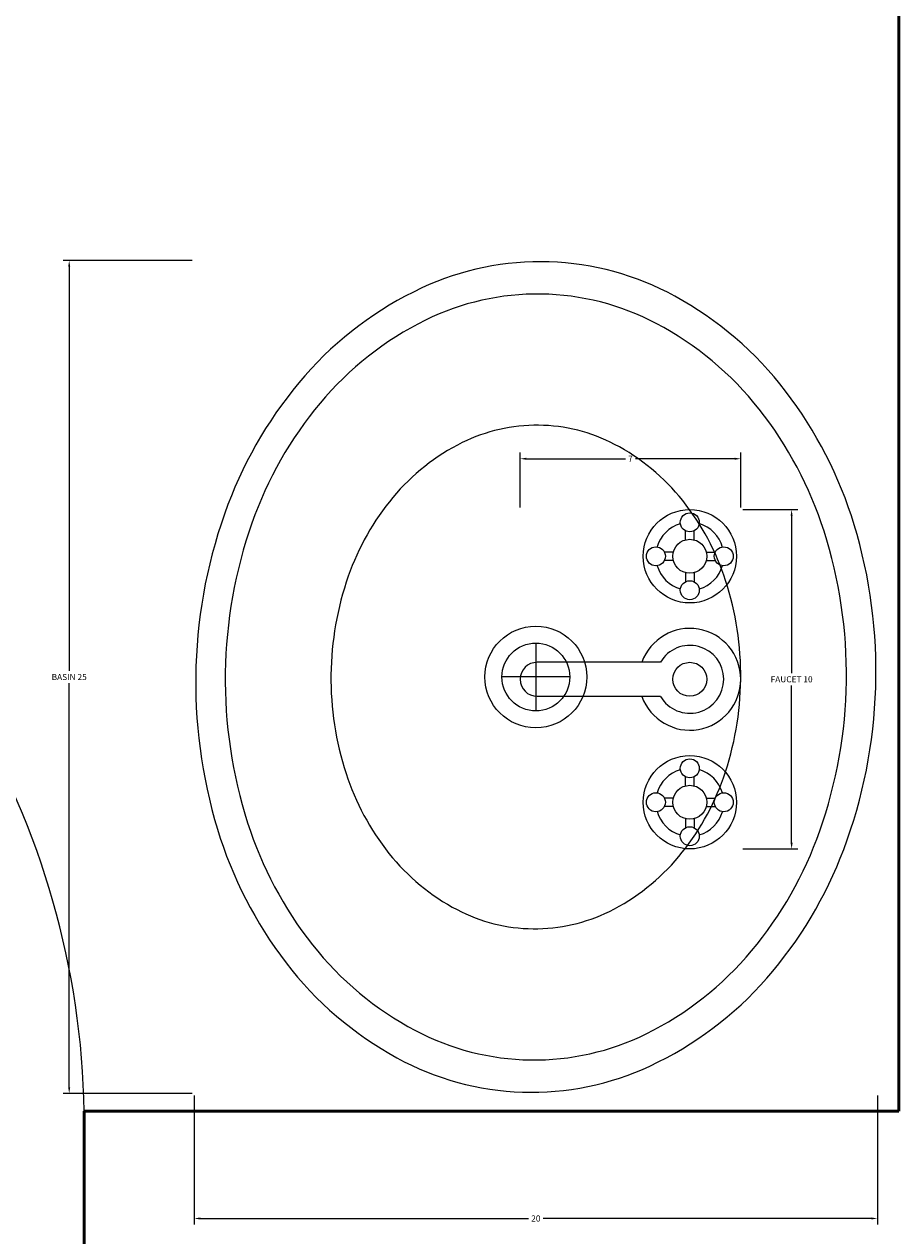
# Model space of a CAD drawing. Units: inches. Extents: x 2621 to 2849, y 2066 to 2463.
# Tile 23 of 28: x 2796 to 2822, y 2372 to 2407. Entities that reach past the tile are written whole.
import ezdxf

# ---------------------------------------------------------------- set-up
doc = ezdxf.new("R2010")
doc.units = ezdxf.units.IN
for name, color, linetype, lineweight in [('A-ANNO-DIMS', 2, 'Continuous', 18), ('A-DOOR', 3, 'Continuous', 25), ('A-FLOR-FIXT', 9, 'Continuous', 18), ('A-WALL', 7, 'Continuous', 50)]:
    doc.layers.add(name, color=color, linetype=linetype, lineweight=lineweight)
doc.styles.get("Standard").update_dxf_attribs({"font": 'arial.ttf'})
doc.dimstyles.get("Standard").update_dxf_attribs({"dimtxt": 0.18, "dimasz": 0.18, "dimexe": 0.18, "dimexo": 0.0625, "dimgap": 0.09, "dimtad": 0, "dimtih": 1, "dimtoh": 1, "dimdec": 4, "dimzin": 0, "dimdsep": 46, "dimtxsty": 'Standard', "dimcen": 0.09, "dimadec": 0, "dimazin": 0, "dimtfac": 1, "dimtdec": 4, "dimtofl": 0, "dimtmove": 0, "dimatfit": 3, "dimfxl": 1, "dimtolj": 1, "dimtzin": 0, "dimarcsym": 0})

# ---------------------------------------------------------------- blocks, each defined once
blk = doc.blocks.new('*U4')
for p, q in [((0, 0), (0, -6)), ((40, 0), (40, -6))]:
    blk.add_line(p, q)
blk.add_lwpolyline([(0, 0), (34.641, 20), (35.516, 18.484), (0.875, -1.516)], close=True)
blk.add_arc((0, 0), 40, 0, 30)
blk = doc.blocks.new('Sink - Oval top')
for p, q in [((0, 1), (0, -1)), ((-1, 0), (1, 0))]:
    blk.add_line(p, q)
for points in [[(-12.234, 0.394, 0.117634), (-11.465, -3.362, 0.104469), (-8.879, -6.804, 0.090016), (-5.083, -9.072, 0.08192), (-0.323, -10.016, 0.08192), (4.488, -9.381, 0.090016), (8.422, -7.361, 0.104469), (11.224, -4.093, 0.117634), (12.234, -0.394, 0.117634), (11.465, 3.362, 0.104469), (8.879, 6.804, 0.090016), (5.083, 9.072, 0.08192), (0.323, 10.016, 0.08192), (-4.488, 9.381, 0.090016), (-8.422, 7.361, 0.104469), (-11.224, 4.093, 0.117634)], [(-11.286, 0.159, 0.118622), (-10.516, -3.253, 0.104678), (-8.072, -6.359, 0.089562), (-4.538, -8.367, 0.081185), (-0.129, -9.152, 0.081185), (4.3, -8.492, 0.089562), (7.889, -6.584, 0.104678), (10.42, -3.548, 0.118622), (11.286, -0.159, 0.118622), (10.516, 3.253, 0.104678), (8.072, 6.359, 0.089562), (4.538, 8.367, 0.081185), (0.129, 9.152, 0.081185), (-4.3, 8.492, 0.089562), (-7.889, 6.584, 0.104678), (-10.42, 3.548, 0.118622)], [(-7.42, 0.083, 0.118283), (-6.907, -2.167, 0.104607), (-5.295, -4.21, 0.089718), (-2.967, -5.528, 0.081436), (-0.068, -6.037, 0.081436), (2.842, -5.593, 0.089718), (5.199, -4.327, 0.104607), (6.857, -2.321, 0.118283), (7.42, -0.083, 0.118283), (6.907, 2.167, 0.104607), (5.295, 4.21, 0.089718), (2.967, 5.528, 0.081436), (0.068, 6.037, 0.081436), (-2.842, 5.593, 0.089718), (-5.199, 4.327, 0.104607), (-6.857, 2.321, 0.118283)]]:
    blk.add_lwpolyline(points, format="xyb", close=True)
for radius in [1.5, 1]:
    blk.add_circle((0, 0), radius)
blk = doc.blocks.new('Faucet - Bathroom top')
for p, q in [((-3.75, 0.4788), (-3.75, 0.75)), ((-3.5, 0.482), (-3.5, 0.75)), ((3.5, 0.4788), (3.5, 0.75)), ((3.75, 0.482), (3.75, 0.75)), ((-4.107, 0.125), (-4.375, 0.125)), ((-3.1461, 0.125), (-2.875, 0.125)), ((3.143, 0.125), (2.875, 0.125)), ((4.1039, 0.125), (4.375, 0.125)), ((-4.1039, -0.125), (-4.375, -0.125)), ((-3.143, -0.125), (-2.875, -0.125)), ((3.1461, -0.125), (2.875, -0.125)), ((4.107, -0.125), (4.375, -0.125)), ((-3.75, -0.4821), (-3.75, -0.75)), ((-3.5, -0.4789), (-3.5, -0.75)), ((3.5, -0.4821), (3.5, -0.75)), ((3.75, -0.4789), (3.75, -0.75)), ((-0.5, -0.8639), (-0.5, -4.5)), ((0.5, -4.5), (0.5, -0.8631))]:
    blk.add_line(p, q)
for centre, radius in [((-3.625, 0), 1.375), ((-3.625, 1), 0.2795), ((3.625, 0), 1.375), ((3.625, 1), 0.2795), ((-3.625, 0), 0.5), ((0, 0), 0.5), ((3.625, 0), 0.5), ((-4.625, 0), 0.2795), ((-2.625, 0), 0.2795), ((2.625, 0), 0.2795), ((4.625, 0), 0.2795), ((-3.625, -1), 0.2795), ((3.625, -1), 0.2795)]:
    blk.add_circle(centre, radius)
for centre, radius, start, end in [((0, 0), 1.5, 289.6514, 250.3603), ((-3.625, 0), 1, 105.2407, 164.2093), ((-3.625, 0), 1, 16.44125, 74.07887), ((0, 0), 1, 300.3431, 239.7554), ((3.625, 0), 1, 106.12, 164.0884), ((3.625, 0), 1, 16.23422, 73.90469), ((-3.625, 0), 1, 196.2342, 253.9047), ((-3.625, 0), 1, 286.12, 344.0884), ((3.625, 0), 1, 196.4413, 254.0789), ((3.625, 0), 1, 285.2407, 344.2093), ((0, -4.5), 0.5, 180, 0)]:
    blk.add_arc(centre, radius, start, end)
blk = doc.blocks.new('*D29')
at = {"layer": 'A-ANNO-DIMS', "color": 0, "lineweight": -2, "transparency": 16777216}
for p, q in [((2801.045, 2400.449), (2797.245, 2400.449)), ((2797.425, 2400.269), (2797.425, 2388.357)), ((2797.425, 2376.078), (2797.425, 2387.99)), ((2801.045, 2375.898), (2797.245, 2375.898))]:
    blk.add_line(p, q, dxfattribs=at)
at = {"layer": 'A-ANNO-DIMS', "color": 0, "transparency": 16777216}
for points in [[(2797.395, 2400.269), (2797.455, 2400.269), (2797.425, 2400.449)], [(2797.395, 2376.078), (2797.455, 2376.078), (2797.425, 2375.898)]]:
    blk.add_solid(points, dxfattribs=at)
at = {"layer": 'Defpoints', "color": 0, "transparency": 16777216}
for p in [(2801.108, 2400.449), (2797.425, 2375.898), (2801.108, 2375.898)]:
    blk.add_point(p, dxfattribs=at)
at = {"layer": 'A-ANNO-DIMS', "color": 0, "transparency": 16777216, "insert": (2797.425, 2388.173), "char_height": 0.18, "attachment_point": 5}
blk.add_mtext('\\A1;BASIN 25', dxfattribs=at)
blk = doc.blocks.new('*D30')
at = {"layer": 'A-ANNO-DIMS', "color": 0, "lineweight": -2, "transparency": 16777216}
for p, q in [((2801.108, 2375.835), (2801.108, 2372.035)), ((2821.244, 2375.835), (2821.244, 2372.035)), ((2801.288, 2372.215), (2810.956, 2372.215)), ((2821.064, 2372.215), (2811.396, 2372.215))]:
    blk.add_line(p, q, dxfattribs=at)
at = {"layer": 'A-ANNO-DIMS', "color": 0, "transparency": 16777216}
for points in [[(2801.288, 2372.245), (2801.288, 2372.185), (2801.108, 2372.215)], [(2821.064, 2372.245), (2821.064, 2372.185), (2821.244, 2372.215)]]:
    blk.add_solid(points, dxfattribs=at)
at = {"layer": 'Defpoints', "color": 0, "transparency": 16777216}
for p in [(2801.108, 2375.898), (2821.244, 2375.898), (2821.244, 2372.215)]:
    blk.add_point(p, dxfattribs=at)
at = {"layer": 'A-ANNO-DIMS', "color": 0, "transparency": 16777216, "insert": (2811.176, 2372.215), "char_height": 0.18, "attachment_point": 5}
blk.add_mtext('\\A1;20', dxfattribs=at)
blk = doc.blocks.new('*D31')
at = {"layer": 'A-ANNO-DIMS', "color": 0, "lineweight": -2, "transparency": 16777216}
for p, q in [((2817.275, 2393.106), (2818.893, 2393.106)), ((2818.713, 2392.926), (2818.713, 2388.289)), ((2818.713, 2383.286), (2818.713, 2387.923)), ((2817.275, 2383.106), (2818.893, 2383.106))]:
    blk.add_line(p, q, dxfattribs=at)
at = {"layer": 'A-ANNO-DIMS', "color": 0, "transparency": 16777216}
for points in [[(2818.683, 2392.926), (2818.743, 2392.926), (2818.713, 2393.106)], [(2818.683, 2383.286), (2818.743, 2383.286), (2818.713, 2383.106)]]:
    blk.add_solid(points, dxfattribs=at)
at = {"layer": 'Defpoints', "color": 0, "transparency": 16777216}
for p in [(2817.213, 2393.106), (2817.213, 2383.106), (2818.713, 2383.106)]:
    blk.add_point(p, dxfattribs=at)
at = {"layer": 'A-ANNO-DIMS', "color": 0, "transparency": 16777216, "insert": (2818.713, 2388.106), "char_height": 0.18, "attachment_point": 5}
blk.add_mtext('\\A1;FAUCET 10', dxfattribs=at)
blk = doc.blocks.new('*D32')
at = {"layer": 'A-ANNO-DIMS', "color": 0, "lineweight": -2, "transparency": 16777216}
for p, q in [((2810.713, 2393.168), (2810.713, 2394.786)), ((2810.893, 2394.606), (2813.815, 2394.606)), ((2817.033, 2394.606), (2814.111, 2394.606)), ((2817.213, 2393.168), (2817.213, 2394.786))]:
    blk.add_line(p, q, dxfattribs=at)
at = {"layer": 'A-ANNO-DIMS', "color": 0, "transparency": 16777216}
for points in [[(2810.893, 2394.636), (2810.893, 2394.576), (2810.713, 2394.606)], [(2817.033, 2394.636), (2817.033, 2394.576), (2817.213, 2394.606)]]:
    blk.add_solid(points, dxfattribs=at)
at = {"layer": 'Defpoints', "color": 0, "transparency": 16777216}
for p in [(2817.213, 2394.606), (2810.713, 2393.106), (2817.213, 2393.106)]:
    blk.add_point(p, dxfattribs=at)
at = {"layer": 'A-ANNO-DIMS', "color": 0, "transparency": 16777216, "insert": (2813.963, 2394.606), "char_height": 0.18, "attachment_point": 5}
blk.add_mtext('\\A1;7', dxfattribs=at)

msp = doc.modelspace()

# ---------------------------------------------------------------- linework, layer by layer
at = {"layer": 'A-WALL'}
for p, q in [((2821.8701, 2435.3746), (2821.8701, 2375.3746)), ((2821.8701, 2435.3746), (2821.8701, 2375.3746)), ((2797.8701, 2375.3746), (2797.8701, 2371.3746)), ((2797.8701, 2375.3746), (2821.8701, 2375.3746))]:
    msp.add_line(p, q, dxfattribs=at)

# ---------------------------------------------------------------- block references
at = {"layer": 'A-DOOR', "xscale": 0.6, "yscale": 0.6, "zscale": 0.6}
msp.add_blockref('*U4', (2773.8701, 2374.9746), dxfattribs=at)
at = {"layer": 'A-FLOR-FIXT', "rotation": 270}
for name, p in [('Sink - Oval top', (2811.176, 2388.1734)), ('Faucet - Bathroom top', (2815.7128, 2388.1058))]:
    msp.add_blockref(name, p, dxfattribs=at)

# ---------------------------------------------------------------- dimensions: what is measured, and where the dimension line sits
at = {"layer": 'A-ANNO-DIMS'}
for base, p1, p2, text, picture, middle in [((2797.4251, 2375.898), (2801.1077, 2400.4489), (2801.1077, 2375.898), 'BASIN <>', '*D29', (2797.4251, 2388.1734)), ((2818.7129, 2383.1058), (2817.2129, 2393.1058), (2817.2129, 2383.1058), 'FAUCET <>', '*D31', (2818.7129, 2388.1058))]:
    dim = msp.add_linear_dim(base=base, p1=p1, p2=p2, angle=270, text=text, dimstyle='Standard', override={"dimdec": 0, "dimlfac": 1, "dimrnd": 0, "dimzin": 0, "dimdsep": 46, "dimlunit": 2}, dxfattribs=at)
    dim.commit()
    dim.dimension.update_dxf_attribs({"geometry": picture, "text_midpoint": middle})
for base, p1, p2, picture, middle in [((2817.2129, 2394.6058), (2810.7128, 2393.1058), (2817.2129, 2393.1058), '*D32', (2813.9629, 2394.6058)), ((2821.2443, 2372.2154), (2801.1077, 2375.898), (2821.2443, 2375.898), '*D30', (2811.176, 2372.2154))]:
    dim = msp.add_linear_dim(base=base, p1=p1, p2=p2, dimstyle='Standard', override={"dimdec": 0, "dimlfac": 1, "dimrnd": 0, "dimzin": 0, "dimdsep": 46, "dimlunit": 2}, dxfattribs=at)
    dim.commit()
    dim.dimension.update_dxf_attribs({"geometry": picture, "text_midpoint": middle})

doc.saveas('drawing.dxf')
